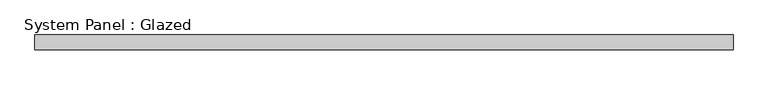
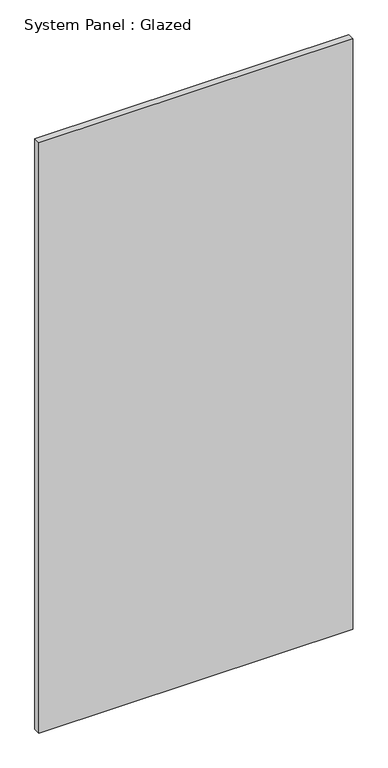
"""IFC4 building model written with IfcOpenShell, lengths in millimetres: plate geometry, System Panel : Glazed."""

from ifc_helpers import new_model, si_unit, origin, origin_with_axes, place, context, project, spatial, polyline, outline, extrude, source, transform, mapped, element, save


def system_panel_glazed_e38def25(model_context):
    return source(origin(), model_context, "Body", "SweptSolid", [
        extrude(outline(polyline([(597.5350001, 19.05), (-597.5350001, 19.05), (-597.5350001, 44.45), (597.5350001, 44.45), (597.5350001, 19.05)])), origin_with_axes(), (0.0, 0.0, 1.0), 2374.9),
    ])


if __name__ == "__main__":
    model = new_model("IFC4")
    model_context = context("Model", 3, world=origin())
    ifc_project = project(units=[si_unit("LENGTHUNIT", "METRE", prefix="MILLI")], contexts=[model_context])
    site = spatial("IfcSite", under=ifc_project)
    building = spatial("IfcBuilding", under=site)
    placement = place(None, origin())
    system_panel_glazed_shape = system_panel_glazed_e38def25(model_context)
    element("IfcPlate", 1, ObjectType="System Panel : Glazed", at=placement, inside=building, context=model_context, shape_type="MappedRepresentation", body=[
        mapped(system_panel_glazed_shape, transform((0.0, 0.0, 0.0), x_axis=(1.0, 0.0, 0.0), y_axis=(0.0, 1.0, 0.0), z_axis=(0.0, 0.0, 1.0))),
    ])
    save(model, "model.ifc")

# Revit data of these elements
# Type "System Panel : Glazed"
#   Construction Type Id = "GSP4R"
#   Analytic Construction = "1/8 in Pilkington single glazing"
#   Visual Light Transmittance = 0.9
#   Solar Heat Gain Coefficient = 0.86
#   Heat Transfer Coefficient (U) = 1.18115 BTU/(h·ft²·°F)
#   Define Thermal Properties by = 1
# Element 1 (IfcPlate, "System Panel : Glazed")
#   Materials on its faces: "Glass"
# Materials
#   "Glass": class "Glass", colour RGB 0 128 192, transparency 0.75, Description = "Soda Lime Glass", Cost = 0
